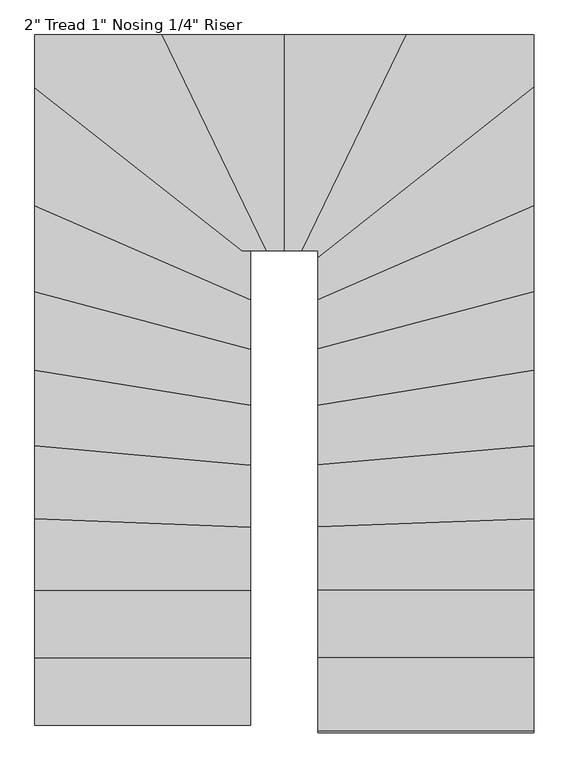
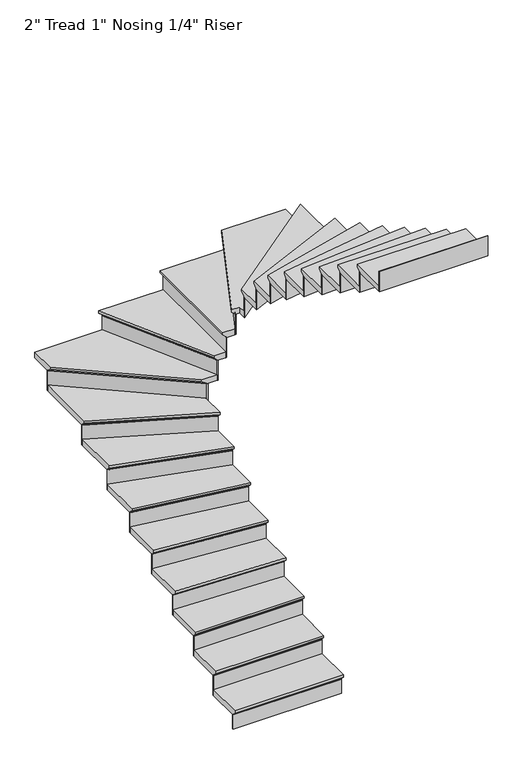
"""IFC4 building model written with IfcOpenShell, lengths in millimetres: stair flight geometry."""

from ifc_helpers import new_model, si_unit, origin, place, context, project, spatial, faceted_brep, source, transform, mapped, element, save


def stair_flight_6c5b5e9d(model_context):
    return source(origin(), model_context, "Body", "Brep", [
        faceted_brep([(-5047.1987704, -4554.2130548, 29415.9214286), (-5047.1987704, -4554.2130548, 29434.9714286), (-5940.8822214, -4554.2130548, 29434.9714286), (-5940.8822214, -4554.2130548, 29415.9214286), (-5047.1987704, -4528.8130548, 29390.5214286), (-5940.8822214, -4528.8130548, 29390.5214286), (-5047.1987704, -4249.4130548, 29434.9714286), (-5940.8822214, -4249.4130548, 29434.9714286), (-5940.8822214, -4528.8130548, 29384.1714286), (-5940.8822214, -4249.4130548, 29384.1714286), (-5047.1987704, -4249.4130548, 29384.1714286), (-5047.1987704, -4528.8130548, 29384.1714286)], [[[0, 1, 2, 3]], [[4, 0, 3, 5]], [[2, 1, 6, 7]], [[8, 9, 10, 11]], [[2, 7, 9, 8, 5, 3]], [[8, 11, 4, 5]], [[6, 1, 0, 4, 11, 10]], [[7, 6, 10, 9]]]),
        faceted_brep([(-5047.1987704, -4528.8130548, 29384.1714286), (-5047.1987704, -4528.8130548, 29260.8), (-5047.1987704, -4522.4630548, 29260.8), (-5047.1987704, -4522.4630548, 29384.1714286), (-5940.8822214, -4528.8130548, 29384.1714286), (-5940.8822214, -4522.4630548, 29384.1714286), (-5940.8822214, -4522.4630548, 29260.8), (-5940.8822214, -4528.8130548, 29260.8)], [[[0, 1, 2, 3]], [[4, 5, 6, 7]], [[1, 0, 4, 7]], [[2, 1, 7, 6]], [[3, 2, 6, 5]], [[0, 3, 5, 4]]]),
        faceted_brep([(-5047.1987704, -4249.4130548, 29558.3428571), (-5047.1987704, -4249.4130548, 29384.1714286), (-5047.1987704, -4243.0630548, 29384.1714286), (-5047.1987704, -4243.0630548, 29558.3428571), (-5940.8822214, -4249.4130548, 29558.3428571), (-5940.8822214, -4243.0630548, 29558.3428571), (-5940.8822214, -4243.0630548, 29384.1714286), (-5940.8822214, -4249.4130548, 29384.1714286)], [[[0, 1, 2, 3]], [[4, 5, 6, 7]], [[1, 0, 4, 7]], [[2, 1, 7, 6]], [[3, 2, 6, 5]], [[0, 3, 5, 4]]]),
        faceted_brep([(-5940.8822214, -4274.8130548, 29609.1428571), (-5047.1987704, -4274.8130548, 29609.1428571), (-5047.1987704, -3970.0130548, 29609.1428571), (-5940.8822214, -3970.0130548, 29609.1428571), (-5940.8822214, -4249.4130548, 29558.3428571), (-5940.8822214, -3970.0130548, 29558.3428571), (-5047.1987704, -3970.0130548, 29558.3428571), (-5047.1987704, -4249.4130548, 29558.3428571), (-5940.8822214, -4249.4130548, 29564.6928571), (-5940.8822214, -4274.8130548, 29590.0928571), (-5047.1987704, -4249.4130548, 29564.6928571), (-5047.1987704, -4274.8130548, 29590.0928571)], [[[0, 1, 2, 3]], [[4, 5, 6, 7]], [[0, 3, 5, 4, 8, 9]], [[4, 7, 10, 8]], [[2, 1, 11, 10, 7, 6]], [[3, 2, 6, 5]], [[11, 1, 0, 9]], [[10, 11, 9, 8]]]),
        faceted_brep([(-5047.1987704, -3970.0130548, 29732.5142857), (-5047.1987704, -3970.0130548, 29558.3428571), (-5047.1987704, -3963.6630548, 29558.3428571), (-5047.1987704, -3963.6630548, 29732.5142857), (-5940.8822214, -3970.0130548, 29732.5142857), (-5940.8822214, -3963.6630548, 29732.5142857), (-5940.8822214, -3963.6630548, 29558.3428571), (-5940.8822214, -3970.0130548, 29558.3428571)], [[[0, 1, 2, 3]], [[4, 5, 6, 7]], [[1, 0, 4, 7]], [[2, 1, 7, 6]], [[3, 2, 6, 5]], [[0, 3, 5, 4]]]),
        faceted_brep([(-5940.8822214, -3995.4130548, 29783.3142857), (-5047.1987704, -3995.4130548, 29783.3142857), (-5047.1987704, -3707.9036879, 29783.3142857), (-5940.8822214, -3673.2843203, 29783.3142857), (-5940.8822214, -3970.0130548, 29732.5142857), (-5940.8822214, -3673.2843203, 29732.5142857), (-5047.1987704, -3707.9036879, 29732.5142857), (-5047.1987704, -3970.0130548, 29732.5142857), (-5940.8822214, -3970.0130548, 29738.8642857), (-5940.8822214, -3995.4130548, 29764.2642857), (-5047.1987704, -3970.0130548, 29738.8642857), (-5047.1987704, -3995.4130548, 29764.2642857)], [[[0, 1, 2, 3]], [[4, 5, 6, 7]], [[0, 3, 5, 4, 8, 9]], [[4, 7, 10, 8]], [[2, 1, 11, 10, 7, 6]], [[3, 2, 6, 5]], [[11, 1, 0, 9]], [[10, 11, 9, 8]]]),
        faceted_brep([(-5047.1987704, -3707.9036879, 29906.6857143), (-5047.1987704, -3707.9036879, 29732.5142857), (-5047.1987704, -3701.5489252, 29732.5142857), (-5047.1987704, -3701.5489252, 29906.6857143), (-5940.8822214, -3673.2843203, 29906.6857143), (-5940.8822214, -3666.9295576, 29906.6857143), (-5940.8822214, -3666.9295576, 29732.5142857), (-5940.8822214, -3673.2843203, 29732.5142857)], [[[0, 1, 2, 3]], [[4, 5, 6, 7]], [[1, 0, 4, 7]], [[2, 1, 7, 6]], [[3, 2, 6, 5]], [[0, 3, 5, 4]]]),
        faceted_brep([(-5940.8822214, -3698.703371, 29957.4857143), (-5047.1987704, -3733.3227386, 29957.4857143), (-5047.1987704, -3451.3234819, 29957.4857143), (-5940.8822214, -3370.89733, 29957.4857143), (-5940.8822214, -3673.2843203, 29906.6857143), (-5940.8822214, -3370.89733, 29906.6857143), (-5047.1987704, -3451.3234819, 29906.6857143), (-5047.1987704, -3707.9036879, 29906.6857143), (-5940.8822214, -3673.2843203, 29913.0357143), (-5940.8822214, -3698.703371, 29938.4357143), (-5047.1987704, -3707.9036879, 29913.0357143), (-5047.1987704, -3733.3227386, 29938.4357143)], [[[0, 1, 2, 3]], [[4, 5, 6, 7]], [[0, 3, 5, 4, 8, 9]], [[4, 7, 10, 8]], [[2, 1, 11, 10, 7, 6]], [[3, 2, 6, 5]], [[11, 1, 0, 9]], [[10, 11, 9, 8]]]),
        faceted_brep([(-5047.1987704, -3451.3234819, 30080.8571429), (-5047.1987704, -3451.3234819, 29906.6857143), (-5047.1987704, -3444.9478197, 29906.6857143), (-5047.1987704, -3444.9478197, 30080.8571429), (-5940.8822214, -3370.89733, 30080.8571429), (-5940.8822214, -3364.5216678, 30080.8571429), (-5940.8822214, -3364.5216678, 29906.6857143), (-5940.8822214, -3370.89733, 29906.6857143)], [[[0, 1, 2, 3]], [[4, 5, 6, 7]], [[1, 0, 4, 7]], [[2, 1, 7, 6]], [[3, 2, 6, 5]], [[0, 3, 5, 4]]]),
        faceted_brep([(-5940.8822214, -3396.3999789, 30131.6571429), (-5047.1987704, -3476.8261308, 30131.6571429), (-5047.1987704, -3203.4301079, 30131.6571429), (-5940.8822214, -3059.5417727, 30131.6571429), (-5940.8822214, -3370.89733, 30080.8571429), (-5940.8822214, -3059.5417727, 30080.8571429), (-5047.1987704, -3203.4301079, 30080.8571429), (-5047.1987704, -3451.3234819, 30080.8571429), (-5940.8822214, -3370.89733, 30087.2071429), (-5940.8822214, -3396.3999789, 30112.6071429), (-5047.1987704, -3451.3234819, 30087.2071429), (-5047.1987704, -3476.8261308, 30112.6071429)], [[[0, 1, 2, 3]], [[4, 5, 6, 7]], [[0, 3, 5, 4, 8, 9]], [[4, 7, 10, 8]], [[2, 1, 11, 10, 7, 6]], [[3, 2, 6, 5]], [[11, 1, 0, 9]], [[10, 11, 9, 8]]]),
        faceted_brep([(-5047.1987704, -3203.4301079, 30255.0285714), (-5047.1987704, -3203.4301079, 30080.8571429), (-5047.1987704, -3196.9983292, 30080.8571429), (-5047.1987704, -3196.9983292, 30255.0285714), (-5940.8822214, -3059.5417727, 30255.0285714), (-5940.8822214, -3053.109994, 30255.0285714), (-5940.8822214, -3053.109994, 30080.8571429), (-5940.8822214, -3059.5417727, 30080.8571429)], [[[0, 1, 2, 3]], [[4, 5, 6, 7]], [[1, 0, 4, 7]], [[2, 1, 7, 6]], [[3, 2, 6, 5]], [[0, 3, 5, 4]]]),
        faceted_brep([(-5940.8822214, -3085.2688872, 30305.8285714), (-5047.1987704, -3229.1572224, 30305.8285714), (-5047.1987704, -2970.3553609, 30305.8285714), (-5940.8822214, -2732.7052783, 30305.8285714), (-5940.8822214, -3059.5417727, 30255.0285714), (-5940.8822214, -2732.7052783, 30255.0285714), (-5047.1987704, -2970.3553609, 30255.0285714), (-5047.1987704, -3203.4301079, 30255.0285714), (-5940.8822214, -3059.5417727, 30261.3785714), (-5940.8822214, -3085.2688872, 30286.7785714), (-5047.1987704, -3203.4301079, 30261.3785714), (-5047.1987704, -3229.1572224, 30286.7785714)], [[[0, 1, 2, 3]], [[4, 5, 6, 7]], [[0, 3, 5, 4, 8, 9]], [[4, 7, 10, 8]], [[2, 1, 11, 10, 7, 6]], [[3, 2, 6, 5]], [[11, 1, 0, 9]], [[10, 11, 9, 8]]]),
        faceted_brep([(-5047.1987704, -2970.3553609, 30429.2), (-5047.1987704, -2970.3553609, 30255.0285714), (-5047.1987704, -2963.7846771, 30255.0285714), (-5047.1987704, -2963.7846771, 30429.2), (-5940.8822214, -2732.7052783, 30429.2), (-5940.8822214, -2726.1345945, 30429.2), (-5940.8822214, -2726.1345945, 30255.0285714), (-5940.8822214, -2732.7052783, 30255.0285714)], [[[0, 1, 2, 3]], [[4, 5, 6, 7]], [[1, 0, 4, 7]], [[2, 1, 7, 6]], [[3, 2, 6, 5]], [[0, 3, 5, 4]]]),
        faceted_brep([(-5940.8822214, -2758.9880136, 30480.0), (-5047.1987704, -2996.6380961, 30480.0), (-5047.1987704, -2765.8050203, 30480.0), (-5940.8822214, -2375.5896532, 30480.0), (-5940.8822214, -2732.7052783, 30429.2), (-5940.8822214, -2375.5896532, 30429.2), (-5047.1987704, -2765.8050203, 30429.2), (-5047.1987704, -2970.3553609, 30429.2), (-5940.8822214, -2732.7052783, 30435.55), (-5940.8822214, -2758.9880136, 30460.95), (-5047.1987704, -2970.3553609, 30435.55), (-5047.1987704, -2996.6380961, 30460.95)], [[[0, 1, 2, 3]], [[4, 5, 6, 7]], [[0, 3, 5, 4, 8, 9]], [[4, 7, 10, 8]], [[2, 1, 11, 10, 7, 6]], [[3, 2, 6, 5]], [[11, 1, 0, 9]], [[10, 11, 9, 8]]]),
        faceted_brep([(-5047.1987704, -2765.8050203, 30603.3714286), (-5047.1987704, -2765.8050203, 30429.2), (-5047.1987704, -2758.8760908, 30429.2), (-5047.1987704, -2758.8760908, 30603.3714286), (-5940.8822214, -2375.5896532, 30603.3714286), (-5940.8822214, -2368.6607237, 30603.3714286), (-5940.8822214, -2368.6607237, 30429.2), (-5940.8822214, -2375.5896532, 30429.2)], [[[0, 1, 2, 3]], [[4, 5, 6, 7]], [[1, 0, 4, 7]], [[2, 1, 7, 6]], [[3, 2, 6, 5]], [[0, 3, 5, 4]]]),
        faceted_brep([(-5940.8822214, -2403.3053713, 30654.1714286), (-5047.1987704, -2793.5207384, 30654.1714286), (-5047.1987704, -2590.8424524, 30654.1714286), (-5040.8038639, -2590.8424524, 30654.1714286), (-5940.8822214, -1882.1944717, 30654.1714286), (-5940.8822214, -2375.5896532, 30603.3714286), (-5940.8822214, -1882.1944717, 30603.3714286), (-5040.8038639, -2590.8424524, 30603.3714286), (-5047.1987704, -2590.8424524, 30603.3714286), (-5047.1987704, -2765.8050203, 30603.3714286), (-5940.8822214, -2375.5896532, 30609.7214286), (-5940.8822214, -2403.3053713, 30635.1214286), (-5047.1987704, -2765.8050203, 30609.7214286), (-5047.1987704, -2793.5207384, 30635.1214286)], [[[0, 1, 2, 3, 4]], [[5, 6, 7, 8, 9]], [[0, 4, 6, 5, 10, 11]], [[5, 9, 12, 10]], [[2, 1, 13, 12, 9, 8]], [[4, 3, 7, 6]], [[13, 1, 0, 11]], [[12, 13, 11, 10]], [[3, 2, 8, 7]]]),
        faceted_brep([(-5040.8038639, -2590.8424524, 30777.5428571), (-5040.8038639, -2590.8424524, 30603.3714286), (-5030.5387554, -2590.8424524, 30603.3714286), (-5030.5387554, -2590.8424524, 30777.5428571), (-5940.8822214, -1882.1944717, 30777.5428571), (-5940.8822214, -1874.1125661, 30777.5428571), (-5940.8822214, -1874.1125661, 30603.3714286), (-5940.8822214, -1882.1944717, 30603.3714286)], [[[0, 1, 2, 3]], [[4, 5, 6, 7]], [[1, 0, 4, 7]], [[2, 1, 7, 6]], [[3, 2, 6, 5]], [[0, 3, 5, 4]]]),
        faceted_brep([(-5384.6489457, -1697.1590014, 30828.3428571), (-5940.8822214, -1697.1590014, 30828.3428571), (-5940.8822214, -1914.5220945, 30828.3428571), (-5081.8642978, -2590.8424524, 30828.3428571), (-4952.3566185, -2590.8424524, 30828.3428571), (-5940.8822214, -1697.1590014, 30777.5428571), (-5384.6489457, -1697.1590014, 30777.5428571), (-4952.3566185, -2590.8424524, 30777.5428571), (-5040.8038639, -2590.8424524, 30777.5428571), (-5940.8822214, -1882.1944717, 30777.5428571), (-5940.8822214, -1882.1944717, 30783.8928571), (-5940.8822214, -1914.5220945, 30809.2928571), (-5040.8038639, -2590.8424524, 30783.8928571), (-5081.8642978, -2590.8424524, 30809.2928571)], [[[0, 1, 2, 3, 4]], [[5, 6, 7, 8, 9]], [[1, 0, 6, 5]], [[2, 1, 5, 9, 10, 11]], [[9, 8, 12, 10]], [[4, 3, 13, 12, 8, 7]], [[0, 4, 7, 6]], [[13, 3, 2, 11]], [[12, 13, 11, 10]]]),
        faceted_brep([(-4952.3566185, -2590.8424524, 30951.7142857), (-4952.3566185, -2590.8424524, 30777.5428571), (-4945.3027294, -2590.8424524, 30777.5428571), (-4945.3027294, -2590.8424524, 30951.7142857), (-5384.6489457, -1697.1590014, 30951.7142857), (-5377.5950566, -1697.1590014, 30951.7142857), (-5377.5950566, -1697.1590014, 30777.5428571), (-5384.6489457, -1697.1590014, 30777.5428571)], [[[0, 1, 2, 3]], [[4, 5, 6, 7]], [[1, 0, 4, 7]], [[2, 1, 7, 6]], [[3, 2, 6, 5]], [[0, 3, 5, 4]]]),
        faceted_brep([(-5412.8645022, -1697.1590014, 31002.5142857), (-4980.5721749, -2590.8424524, 31002.5142857), (-4882.0987704, -2590.8424524, 31002.5142857), (-4882.0987706, -1697.1590014, 31002.5142857), (-5384.6489457, -1697.1590014, 30951.7142857), (-4882.0987706, -1697.1590014, 30951.7142857), (-4882.0987704, -2590.8424524, 30951.7142857), (-4952.3566185, -2590.8424524, 30951.7142857), (-5384.6489457, -1697.1590014, 30958.0642857), (-5412.8645022, -1697.1590014, 30983.4642857), (-4952.3566185, -2590.8424524, 30958.0642857), (-4980.5721749, -2590.8424524, 30983.4642857)], [[[0, 1, 2, 3]], [[4, 5, 6, 7]], [[0, 3, 5, 4, 8, 9]], [[4, 7, 10, 8]], [[3, 2, 6, 5]], [[11, 1, 0, 9]], [[10, 11, 9, 8]], [[2, 1, 11, 10, 7, 6]]]),
        faceted_brep([(-4882.0987704, -2590.8424524, 31125.8857143), (-4882.0987704, -2590.8424524, 30951.7142857), (-4875.7487704, -2590.8424524, 30951.7142857), (-4875.7487704, -2590.8424524, 31125.8857143), (-4882.0987706, -1697.1590014, 31125.8857143), (-4875.7487706, -1697.1590014, 31125.8857143), (-4875.7487706, -1697.1590014, 30951.7142857), (-4882.0987706, -1697.1590014, 30951.7142857)], [[[0, 1, 2, 3]], [[4, 5, 6, 7]], [[1, 0, 4, 7]], [[2, 1, 7, 6]], [[3, 2, 6, 5]], [[0, 3, 5, 4]]]),
        faceted_brep([(-4907.4987706, -1697.1590014, 31176.6857143), (-4907.4987704, -2590.8424524, 31176.6857143), (-4806.2098095, -2590.8424524, 31176.6857143), (-4373.9174828, -1697.1590014, 31176.6857143), (-4882.0987706, -1697.1590014, 31125.8857143), (-4373.9174828, -1697.1590014, 31125.8857143), (-4806.2098095, -2590.8424524, 31125.8857143), (-4882.0987704, -2590.8424524, 31125.8857143), (-4882.0987706, -1697.1590014, 31132.2357143), (-4907.4987706, -1697.1590014, 31157.6357143), (-4882.0987704, -2590.8424524, 31132.2357143), (-4907.4987704, -2590.8424524, 31157.6357143)], [[[0, 1, 2, 3]], [[4, 5, 6, 7]], [[0, 3, 5, 4, 8, 9]], [[4, 7, 10, 8]], [[2, 1, 11, 10, 7, 6]], [[3, 2, 6, 5]], [[11, 1, 0, 9]], [[10, 11, 9, 8]]]),
        faceted_brep([(-4806.2098095, -2590.8424524, 31300.0571429), (-4806.2098095, -2590.8424524, 31125.8857143), (-4799.1559204, -2590.8424524, 31125.8857143), (-4799.1559204, -2590.8424524, 31300.0571429), (-4373.9174828, -1697.1590014, 31300.0571429), (-4366.8635937, -1697.1590014, 31300.0571429), (-4366.8635937, -1697.1590014, 31125.8857143), (-4373.9174828, -1697.1590014, 31125.8857143)], [[[0, 1, 2, 3]], [[4, 5, 6, 7]], [[1, 0, 4, 7]], [[2, 1, 7, 6]], [[3, 2, 6, 5]], [[0, 3, 5, 4]]]),
        faceted_brep([(-3874.1153195, -1946.8497166, 31350.8571429), (-3874.1153195, -1697.1590014, 31350.8571429), (-4402.1330392, -1697.1590014, 31350.8571429), (-4834.4253659, -2590.8424524, 31350.8571429), (-4767.7987704, -2590.8424524, 31350.8571429), (-4767.7987704, -2650.4628721, 31350.8571429), (-3874.1153195, -1697.1590014, 31300.0571429), (-3874.1153195, -1946.8497166, 31300.0571429), (-4767.7987704, -2650.4628721, 31300.0571429), (-4767.7987704, -2590.8424524, 31300.0571429), (-4806.2098095, -2590.8424524, 31300.0571429), (-4373.9174828, -1697.1590014, 31300.0571429), (-4806.2098095, -2590.8424524, 31306.4071429), (-4373.9174828, -1697.1590014, 31306.4071429), (-4834.4253659, -2590.8424524, 31331.8071429), (-4402.1330392, -1697.1590014, 31331.8071429)], [[[0, 1, 2, 3, 4, 5]], [[6, 7, 8, 9, 10, 11]], [[1, 0, 7, 6]], [[11, 10, 12, 13]], [[4, 3, 14, 12, 10, 9]], [[5, 4, 9, 8]], [[0, 5, 8, 7]], [[14, 3, 2, 15]], [[12, 14, 15, 13]], [[2, 1, 6, 11, 13, 15]]]),
        faceted_brep([(-4767.7987704, -2650.4628721, 31474.2285714), (-4767.7987704, -2650.4628721, 31300.0571429), (-4767.7987704, -2658.5447778, 31300.0571429), (-4767.7987704, -2658.5447778, 31474.2285714), (-3874.1153195, -1946.8497166, 31474.2285714), (-3874.1153195, -1954.9316222, 31474.2285714), (-3874.1153195, -1954.9316222, 31300.0571429), (-3874.1153195, -1946.8497166, 31300.0571429)], [[[0, 1, 2, 3]], [[4, 5, 6, 7]], [[1, 0, 4, 7]], [[2, 1, 7, 6]], [[3, 2, 6, 5]], [[0, 3, 5, 4]]]),
        faceted_brep([(-3874.1153195, -1914.5220938, 31525.0285714), (-4767.7987704, -2618.1352494, 31525.0285714), (-4767.7987704, -2821.2364563, 31525.0285714), (-3874.1153195, -2431.0210889, 31525.0285714), (-3874.1153195, -1946.8497166, 31474.2285714), (-3874.1153195, -2431.0210889, 31474.2285714), (-4767.7987704, -2821.2364563, 31474.2285714), (-4767.7987704, -2650.4628721, 31474.2285714), (-3874.1153195, -1946.8497166, 31480.5785714), (-3874.1153195, -1914.5220938, 31505.9785714), (-4767.7987704, -2650.4628721, 31480.5785714), (-4767.7987704, -2618.1352494, 31505.9785714)], [[[0, 1, 2, 3]], [[4, 5, 6, 7]], [[0, 3, 5, 4, 8, 9]], [[4, 7, 10, 8]], [[2, 1, 11, 10, 7, 6]], [[3, 2, 6, 5]], [[11, 1, 0, 9]], [[10, 11, 9, 8]]]),
        faceted_brep([(-4767.7987704, -2821.2364563, 31648.4), (-4767.7987704, -2821.2364563, 31474.2285714), (-4767.7987704, -2828.1653858, 31474.2285714), (-4767.7987704, -2828.1653858, 31648.4), (-3874.1153195, -2431.0210889, 31648.4), (-3874.1153195, -2437.9500185, 31648.4), (-3874.1153195, -2437.9500185, 31474.2285714), (-3874.1153195, -2431.0210889, 31474.2285714)], [[[0, 1, 2, 3]], [[4, 5, 6, 7]], [[1, 0, 4, 7]], [[2, 1, 7, 6]], [[3, 2, 6, 5]], [[0, 3, 5, 4]]]),
        faceted_brep([(-3874.1153195, -2403.3053709, 31699.2), (-4767.7987704, -2793.5207382, 31699.2), (-4767.7987704, -3022.9208311, 31699.2), (-3874.1153195, -2785.2707484, 31699.2), (-3874.1153195, -2431.0210889, 31648.4), (-3874.1153195, -2785.2707484, 31648.4), (-4767.7987704, -3022.9208311, 31648.4), (-4767.7987704, -2821.2364563, 31648.4), (-3874.1153195, -2431.0210889, 31654.75), (-3874.1153195, -2403.3053709, 31680.15), (-4767.7987704, -2821.2364563, 31654.75), (-4767.7987704, -2793.5207382, 31680.15)], [[[0, 1, 2, 3]], [[4, 5, 6, 7]], [[0, 3, 5, 4, 8, 9]], [[4, 7, 10, 8]], [[2, 1, 11, 10, 7, 6]], [[3, 2, 6, 5]], [[11, 1, 0, 9]], [[10, 11, 9, 8]]]),
        faceted_brep([(-4767.7987704, -3022.9208311, 31822.5714286), (-4767.7987704, -3022.9208311, 31648.4), (-4767.7987704, -3029.4915149, 31648.4), (-4767.7987704, -3029.4915149, 31822.5714286), (-3874.1153195, -2785.2707484, 31822.5714286), (-3874.1153195, -2791.8414322, 31822.5714286), (-3874.1153195, -2791.8414322, 31648.4), (-3874.1153195, -2785.2707484, 31648.4)], [[[0, 1, 2, 3]], [[4, 5, 6, 7]], [[1, 0, 4, 7]], [[2, 1, 7, 6]], [[3, 2, 6, 5]], [[0, 3, 5, 4]]]),
        faceted_brep([(-3874.1153195, -2758.9880132, 31873.3714286), (-4767.7987704, -2996.6380959, 31873.3714286), (-4767.7987704, -3254.8843368, 31873.3714286), (-3874.1153195, -3110.9960015, 31873.3714286), (-3874.1153195, -2785.2707484, 31822.5714286), (-3874.1153195, -3110.9960015, 31822.5714286), (-4767.7987704, -3254.8843368, 31822.5714286), (-4767.7987704, -3022.9208311, 31822.5714286), (-3874.1153195, -2785.2707484, 31828.9214286), (-3874.1153195, -2758.9880132, 31854.3214286), (-4767.7987704, -3022.9208311, 31828.9214286), (-4767.7987704, -2996.6380959, 31854.3214286)], [[[0, 1, 2, 3]], [[4, 5, 6, 7]], [[0, 3, 5, 4, 8, 9]], [[4, 7, 10, 8]], [[2, 1, 11, 10, 7, 6]], [[3, 2, 6, 5]], [[11, 1, 0, 9]], [[10, 11, 9, 8]]]),
        faceted_brep([(-4767.7987704, -3254.8843368, 31996.7428571), (-4767.7987704, -3254.8843368, 31822.5714286), (-4767.7987704, -3261.3161154, 31822.5714286), (-4767.7987704, -3261.3161154, 31996.7428571), (-3874.1153195, -3110.9960015, 31996.7428571), (-3874.1153195, -3117.4277801, 31996.7428571), (-3874.1153195, -3117.4277801, 31822.5714286), (-3874.1153195, -3110.9960015, 31822.5714286)], [[[0, 1, 2, 3]], [[4, 5, 6, 7]], [[1, 0, 4, 7]], [[2, 1, 7, 6]], [[3, 2, 6, 5]], [[0, 3, 5, 4]]]),
        faceted_brep([(-3874.1153195, -3085.2688869, 32047.5428571), (-4767.7987704, -3229.1572222, 32047.5428571), (-4767.7987704, -3502.3287795, 32047.5428571), (-3874.1153195, -3421.9026274, 32047.5428571), (-3874.1153195, -3110.9960015, 31996.7428571), (-3874.1153195, -3421.9026274, 31996.7428571), (-4767.7987704, -3502.3287795, 31996.7428571), (-4767.7987704, -3254.8843368, 31996.7428571), (-3874.1153195, -3110.9960015, 32003.0928571), (-3874.1153195, -3085.2688869, 32028.4928571), (-4767.7987704, -3254.8843368, 32003.0928571), (-4767.7987704, -3229.1572222, 32028.4928571)], [[[0, 1, 2, 3]], [[4, 5, 6, 7]], [[0, 3, 5, 4, 8, 9]], [[4, 7, 10, 8]], [[2, 1, 11, 10, 7, 6]], [[3, 2, 6, 5]], [[11, 1, 0, 9]], [[10, 11, 9, 8]]]),
        faceted_brep([(-4767.7987704, -3502.3287795, 32170.9142857), (-4767.7987704, -3502.3287795, 31996.7428571), (-4767.7987704, -3508.7044417, 31996.7428571), (-4767.7987704, -3508.7044417, 32170.9142857), (-3874.1153195, -3421.9026274, 32170.9142857), (-3874.1153195, -3428.2782897, 32170.9142857), (-3874.1153195, -3428.2782897, 31996.7428571), (-3874.1153195, -3421.9026274, 31996.7428571)], [[[0, 1, 2, 3]], [[4, 5, 6, 7]], [[1, 0, 4, 7]], [[2, 1, 7, 6]], [[3, 2, 6, 5]], [[0, 3, 5, 4]]]),
        faceted_brep([(-3874.1153195, -3396.3999786, 32221.7142857), (-4767.7987704, -3476.8261306, 32221.7142857), (-4767.7987704, -3758.7417891, 32221.7142857), (-3874.1153195, -3724.1224215, 32221.7142857), (-3874.1153195, -3421.9026274, 32170.9142857), (-3874.1153195, -3724.1224215, 32170.9142857), (-4767.7987704, -3758.7417891, 32170.9142857), (-4767.7987704, -3502.3287795, 32170.9142857), (-3874.1153195, -3421.9026274, 32177.2642857), (-3874.1153195, -3396.3999786, 32202.6642857), (-4767.7987704, -3502.3287795, 32177.2642857), (-4767.7987704, -3476.8261306, 32202.6642857)], [[[0, 1, 2, 3]], [[4, 5, 6, 7]], [[0, 3, 5, 4, 8, 9]], [[4, 7, 10, 8]], [[2, 1, 11, 10, 7, 6]], [[3, 2, 6, 5]], [[11, 1, 0, 9]], [[10, 11, 9, 8]]]),
        faceted_brep([(-4767.7987704, -3758.7417891, 32345.0857143), (-4767.7987704, -3758.7417891, 32170.9142857), (-4767.7987704, -3765.0965518, 32170.9142857), (-4767.7987704, -3765.0965518, 32345.0857143), (-3874.1153195, -3724.1224215, 32345.0857143), (-3874.1153195, -3730.4771842, 32345.0857143), (-3874.1153195, -3730.4771842, 32170.9142857), (-3874.1153195, -3724.1224215, 32170.9142857)], [[[0, 1, 2, 3]], [[4, 5, 6, 7]], [[1, 0, 4, 7]], [[2, 1, 7, 6]], [[3, 2, 6, 5]], [[0, 3, 5, 4]]]),
        faceted_brep([(-3874.1153195, -3698.7033708, 32395.8857143), (-4767.7987704, -3733.3227384, 32395.8857143), (-4767.7987704, -4020.8130546, 32395.8857143), (-3874.1153195, -4020.8130546, 32395.8857143), (-3874.1153195, -3724.1224215, 32345.0857143), (-3874.1153195, -4020.8130546, 32345.0857143), (-4767.7987704, -4020.8130546, 32345.0857143), (-4767.7987704, -3758.7417891, 32345.0857143), (-3874.1153195, -3724.1224215, 32351.4357143), (-3874.1153195, -3698.7033708, 32376.8357143), (-4767.7987704, -3758.7417891, 32351.4357143), (-4767.7987704, -3733.3227384, 32376.8357143)], [[[0, 1, 2, 3]], [[4, 5, 6, 7]], [[0, 3, 5, 4, 8, 9]], [[4, 7, 10, 8]], [[2, 1, 11, 10, 7, 6]], [[3, 2, 6, 5]], [[11, 1, 0, 9]], [[10, 11, 9, 8]]]),
        faceted_brep([(-4767.7987704, -4020.8130546, 32519.2571429), (-4767.7987704, -4020.8130546, 32345.0857143), (-4767.7987704, -4027.1630546, 32345.0857143), (-4767.7987704, -4027.1630546, 32519.2571429), (-3874.1153195, -4020.8130546, 32519.2571429), (-3874.1153195, -4027.1630546, 32519.2571429), (-3874.1153195, -4027.1630546, 32345.0857143), (-3874.1153195, -4020.8130546, 32345.0857143)], [[[0, 1, 2, 3]], [[4, 5, 6, 7]], [[1, 0, 4, 7]], [[2, 1, 7, 6]], [[3, 2, 6, 5]], [[0, 3, 5, 4]]]),
        faceted_brep([(-3874.1153195, -3995.4130546, 32570.0571429), (-4767.7987704, -3995.4130546, 32570.0571429), (-4767.7987704, -4300.2130546, 32570.0571429), (-3874.1153195, -4300.2130546, 32570.0571429), (-3874.1153195, -4020.8130546, 32519.2571429), (-3874.1153195, -4300.2130546, 32519.2571429), (-4767.7987704, -4300.2130546, 32519.2571429), (-4767.7987704, -4020.8130546, 32519.2571429), (-3874.1153195, -4020.8130546, 32525.6071429), (-3874.1153195, -3995.4130546, 32551.0071429), (-4767.7987704, -4020.8130546, 32525.6071429), (-4767.7987704, -3995.4130546, 32551.0071429)], [[[0, 1, 2, 3]], [[4, 5, 6, 7]], [[0, 3, 5, 4, 8, 9]], [[4, 7, 10, 8]], [[2, 1, 11, 10, 7, 6]], [[3, 2, 6, 5]], [[11, 1, 0, 9]], [[10, 11, 9, 8]]]),
        faceted_brep([(-4767.7987704, -4300.2130546, 32693.4285714), (-4767.7987704, -4300.2130546, 32519.2571429), (-4767.7987704, -4306.5630546, 32519.2571429), (-4767.7987704, -4306.5630546, 32693.4285714), (-3874.1153195, -4300.2130546, 32693.4285714), (-3874.1153195, -4306.5630546, 32693.4285714), (-3874.1153195, -4306.5630546, 32519.2571429), (-3874.1153195, -4300.2130546, 32519.2571429)], [[[0, 1, 2, 3]], [[4, 5, 6, 7]], [[1, 0, 4, 7]], [[2, 1, 7, 6]], [[3, 2, 6, 5]], [[0, 3, 5, 4]]]),
        faceted_brep([(-4767.7987704, -4579.6130546, 32867.6), (-4767.7987704, -4579.6130546, 32693.4285714), (-4767.7987704, -4585.9630546, 32693.4285714), (-4767.7987704, -4585.9630546, 32867.6), (-3874.1153195, -4579.6130546, 32867.6), (-3874.1153195, -4585.9630546, 32867.6), (-3874.1153195, -4585.9630546, 32693.4285714), (-3874.1153195, -4579.6130546, 32693.4285714)], [[[0, 1, 2, 3]], [[4, 5, 6, 7]], [[1, 0, 4, 7]], [[2, 1, 7, 6]], [[3, 2, 6, 5]], [[0, 3, 5, 4]]]),
        faceted_brep([(-3874.1153195, -4274.8130546, 32744.2285714), (-4767.7987704, -4274.8130546, 32744.2285714), (-4767.7987704, -4579.6130546, 32744.2285714), (-3874.1153195, -4579.6130546, 32744.2285714), (-3874.1153195, -4300.2130546, 32693.4285714), (-3874.1153195, -4579.6130546, 32693.4285714), (-4767.7987704, -4579.6130546, 32693.4285714), (-4767.7987704, -4300.2130546, 32693.4285714), (-3874.1153195, -4300.2130546, 32699.7785714), (-3874.1153195, -4274.8130546, 32725.1785714), (-4767.7987704, -4300.2130546, 32699.7785714), (-4767.7987704, -4274.8130546, 32725.1785714)], [[[0, 1, 2, 3]], [[4, 5, 6, 7]], [[0, 3, 5, 4, 8, 9]], [[4, 7, 10, 8]], [[2, 1, 11, 10, 7, 6]], [[3, 2, 6, 5]], [[11, 1, 0, 9]], [[10, 11, 9, 8]]]),
    ])


if __name__ == "__main__":
    model = new_model("IFC4")
    model_context = context("Model", 3, world=origin())
    ifc_project = project(units=[si_unit("LENGTHUNIT", "METRE", prefix="MILLI")], contexts=[model_context])
    site = spatial("IfcSite", under=ifc_project)
    building = spatial("IfcBuilding", under=site)
    placement = place(None, origin())
    stair_flight_shape = stair_flight_6c5b5e9d(model_context)
    element("IfcStairFlight", 1, ObjectType="2\" Tread 1\" Nosing 1/4\" Riser", at=placement, inside=building, context=model_context, shape_type="MappedRepresentation", body=[
        mapped(stair_flight_shape, transform((0.0, 0.0, 0.0), x_axis=(1.0, 0.0, 0.0), y_axis=(0.0, 1.0, 0.0), z_axis=(0.0, 0.0, 1.0))),
    ])
    save(model, "model.ifc")

# Revit data of these elements
# Element 1 (IfcStairFlight, "2\" Tread 1\" Nosing 1/4\" Riser")
#   Materials on its faces: "Tile, Porcelain, 4in"
# Materials
#   "Tile, Porcelain, 4in": class "Generic", colour RGB 89 87 158, transparency 0, Description = "Porcelain tile, 4\", white", Cost = 0
